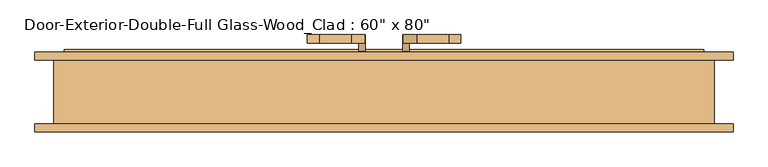
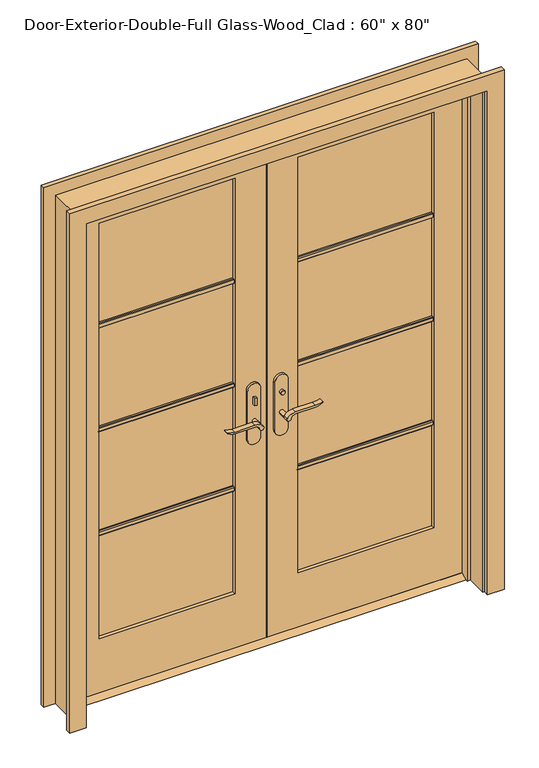
"""IFC4 building model written with IfcOpenShell, lengths in millimetres: door geometry."""

from ifc_helpers import new_model, si_unit, point, frame, frame_2d, origin, place, context, project, spatial, polyline, circle_curve, trimmed, segment, composite_curve, outline, extrude, faceted_brep, source, transform, mapped, element, save


def door_94998e6c(model_context):
    return source(origin(), model_context, "Body", "SolidModel", [
        extrude(outline(polyline([(38.1, 12.7), (73.025, 12.7), (98.425, 0.0), (12.7, 0.0), (38.1, 12.7)])), frame((-762.0, 0.0, 0.0), z_axis=(1.0, 0.0, 0.0), x_axis=(0.0, 1.0, 0.0)), (0.0, 0.0, 1.0), 1524.0),
        extrude(outline(polyline([(-47.4019111, 18.1), (-57.4019111, 18.1), (-57.4019111, 28.1), (-47.4019111, 28.1), (-47.4019111, 18.1)])), frame((0.0, 0.0, 981.9), z_axis=(0.0, 0.0, 1.0), x_axis=(1.0, 0.0, 0.0)), (0.0, 0.0, 1.0), 30.0),
        extrude(outline(composite_curve([segment(trimmed(circle_curve(frame_2d((996.9, -52.4019111)), 8.0), [point((996.9, -60.4019111))], [point((996.9, -44.4019111))], False, "CARTESIAN"), True, "CONTINUOUS"), segment(trimmed(circle_curve(frame_2d((996.9, -52.4019111)), 8.0), [point((996.9, -44.4019111))], [point((996.9, -60.4019111))], False, "CARTESIAN"), True, "CONTINUOUS")], self_intersect=False)), frame((0.0, 83.025, 0.0), z_axis=(0.0, 1.0, 0.0), x_axis=(0.0, 0.0, 1.0)), (0.0, 0.0, 1.0), 10.0),
        extrude(outline(composite_curve([segment(trimmed(circle_curve(frame_2d((897.1555521, -76.0694241)), 37.2832219), [point((919.0523287, -45.8937749))], [point((934.4, -77.7693445))], False, "CARTESIAN"), True, "CONTINUOUS"), segment(polyline([(934.4, -77.7693445), (934.4, -154.045502)]), True, "CONTINUOUS"), segment(trimmed(circle_curve(frame_2d((1017.6850638, -153.9791202)), 83.2850902), [point((934.4, -154.045502))], [point((939.4, -182.4019111))], True, "CARTESIAN"), True, "CONTINUOUS"), segment(polyline([(939.4, -182.4019111), (936.6135558, -182.4019111)]), True, "CONTINUOUS"), segment(trimmed(circle_curve(frame_2d((986.6709207, -150.4622499)), 59.3791355), [point((936.6135558, -182.4019111))], [point((927.4, -154.045502))], False, "CARTESIAN"), True, "CONTINUOUS"), segment(polyline([(927.4, -154.045502), (927.4, -77.7881013)]), True, "CONTINUOUS"), segment(trimmed(circle_curve(frame_2d((909.2738613, -77.7881013)), 18.1261387), [point((927.4, -77.7881013))], [point((914.4, -60.4019111))], True, "CARTESIAN"), True, "CONTINUOUS"), segment(trimmed(circle_curve(frame_2d((914.4, -52.4019111)), 8.0), [point((914.4, -60.4019111))], [point((919.0523287, -45.8937749))], False, "CARTESIAN"), True, "CONTINUOUS")], self_intersect=False)), frame((0.0, -21.9, 0.0), z_axis=(0.0, 1.0, 0.0), x_axis=(0.0, 0.0, 1.0)), (0.0, 0.0, 1.0), 20.0),
        extrude(outline(composite_curve([segment(trimmed(circle_curve(frame_2d((914.4, -52.4019111)), 8.0), [point((914.3999903, -60.4019111))], [point((919.0523287, -45.8937749))], False, "CARTESIAN"), True, "CONTINUOUS"), segment(trimmed(circle_curve(frame_2d((897.1555521, -76.0694241)), 37.2832219), [point((919.0523287, -45.8937749))], [point((934.4, -77.7693445))], False, "CARTESIAN"), True, "CONTINUOUS"), segment(polyline([(934.4, -77.7693445), (934.4, -154.045502)]), True, "CONTINUOUS"), segment(trimmed(circle_curve(frame_2d((1017.6850638, -153.9791202)), 83.2850902), [point((934.4, -154.045502))], [point((939.4, -182.4019111))], True, "CARTESIAN"), True, "CONTINUOUS"), segment(polyline([(939.4, -182.4019111), (936.6135558, -182.4019111)]), True, "CONTINUOUS"), segment(trimmed(circle_curve(frame_2d((986.6709207, -150.4622499)), 59.3791355), [point((936.6135558, -182.4019111))], [point((927.4, -154.045502))], False, "CARTESIAN"), True, "CONTINUOUS"), segment(polyline([(927.4, -154.045502), (927.4, -77.788099)]), True, "CONTINUOUS"), segment(trimmed(circle_curve(frame_2d((909.2738682, -77.788099)), 18.1261318), [point((927.4, -77.788099))], [point((914.3999903, -60.4019111))], True, "CARTESIAN"), True, "CONTINUOUS")], self_intersect=False)), frame((0.0, 113.025, 0.0), z_axis=(0.0, 1.0, 0.0), x_axis=(0.0, 0.0, 1.0)), (0.0, 0.0, 1.0), 20.0),
        extrude(outline(composite_curve([segment(trimmed(circle_curve(frame_2d((914.4, -52.4019111)), 8.0), [point((914.4, -60.4019111))], [point((914.4, -44.4019111))], False, "CARTESIAN"), True, "CONTINUOUS"), segment(trimmed(circle_curve(frame_2d((914.4, -52.4019111)), 8.0), [point((914.4, -44.4019111))], [point((914.4, -60.4019111))], False, "CARTESIAN"), True, "CONTINUOUS")], self_intersect=False)), frame((0.0, -1.9, 0.0), z_axis=(0.0, 1.0, 0.0), x_axis=(0.0, 0.0, 1.0)), (0.0, 0.0, 1.0), 30.0),
        extrude(outline(composite_curve([segment(trimmed(circle_curve(frame_2d((914.4, -52.4019111)), 8.0), [point((914.4, -60.4019111))], [point((914.4, -44.4019111))], False, "CARTESIAN"), True, "CONTINUOUS"), segment(trimmed(circle_curve(frame_2d((914.4, -52.4019111)), 8.0), [point((914.4, -44.4019111))], [point((914.4, -60.4019111))], False, "CARTESIAN"), True, "CONTINUOUS")], self_intersect=False)), frame((0.0, 83.025, 0.0), z_axis=(0.0, 1.0, 0.0), x_axis=(0.0, 0.0, 1.0)), (0.0, 0.0, 1.0), 30.0),
        extrude(outline(composite_curve([segment(polyline([(844.4, -27.4019111), (1039.4, -27.4019111)]), True, "CONTINUOUS"), segment(trimmed(circle_curve(frame_2d((1039.4, -52.4019111)), 25.0), [point((1039.4, -27.4019111))], [point((1039.4, -77.4019111))], False, "CARTESIAN"), True, "CONTINUOUS"), segment(polyline([(1039.4, -77.4019111), (844.4, -77.4019111)]), True, "CONTINUOUS"), segment(trimmed(circle_curve(frame_2d((844.4, -52.4019111)), 25.0), [point((844.4, -77.4019111))], [point((844.4, -27.4019111))], False, "CARTESIAN"), True, "CONTINUOUS")], self_intersect=False)), frame((0.0, 28.1, 0.0), z_axis=(0.0, 1.0, 0.0), x_axis=(0.0, 0.0, 1.0)), (0.0, 0.0, 1.0), 10.0),
        extrude(outline(composite_curve([segment(polyline([(844.4, -27.4019111), (1039.4, -27.4019111)]), True, "CONTINUOUS"), segment(trimmed(circle_curve(frame_2d((1039.4, -52.4019111)), 25.0), [point((1039.4, -27.4019111))], [point((1039.4, -77.4019111))], False, "CARTESIAN"), True, "CONTINUOUS"), segment(polyline([(1039.4, -77.4019111), (844.4, -77.4019111)]), True, "CONTINUOUS"), segment(trimmed(circle_curve(frame_2d((844.4, -52.4019111)), 25.0), [point((844.4, -77.4019111))], [point((844.4, -27.4019111))], False, "CARTESIAN"), True, "CONTINUOUS")], self_intersect=False)), frame((0.0, 73.025, 0.0), z_axis=(0.0, 1.0, 0.0), x_axis=(0.0, 0.0, 1.0)), (0.0, 0.0, 1.0), 10.0),
        extrude(outline(polyline([(47.3875, 93.025), (57.3875, 93.025), (57.3875, 83.025), (47.3875, 83.025), (47.3875, 93.025)])), frame((0.0, 0.0, 981.9), z_axis=(0.0, 0.0, 1.0), x_axis=(1.0, 0.0, 0.0)), (0.0, 0.0, 1.0), 30.0),
        extrude(outline(composite_curve([segment(trimmed(circle_curve(frame_2d((996.9, 52.3875)), 8.0), [point((996.9, 60.3875))], [point((996.9, 44.3875))], False, "CARTESIAN"), True, "CONTINUOUS"), segment(trimmed(circle_curve(frame_2d((996.9, 52.3875)), 8.0), [point((996.9, 44.3875))], [point((996.9, 60.3875))], False, "CARTESIAN"), True, "CONTINUOUS")], self_intersect=False)), frame((0.0, 18.1, 0.0), z_axis=(0.0, 1.0, 0.0), x_axis=(0.0, 0.0, 1.0)), (0.0, 0.0, 1.0), 10.0),
        extrude(outline(composite_curve([segment(trimmed(circle_curve(frame_2d((914.4, 52.3875)), 8.0), [point((919.0523287, 45.8793637))], [point((914.4, 60.3875))], False, "CARTESIAN"), True, "CONTINUOUS"), segment(trimmed(circle_curve(frame_2d((909.2738613, 77.7736901)), 18.1261387), [point((914.4, 60.3875))], [point((927.4, 77.7736901))], True, "CARTESIAN"), True, "CONTINUOUS"), segment(polyline([(927.4, 77.7736901), (927.4, 154.0310909)]), True, "CONTINUOUS"), segment(trimmed(circle_curve(frame_2d((986.6709207, 150.4478388)), 59.3791355), [point((927.4, 154.0310909))], [point((936.6135558, 182.3875))], False, "CARTESIAN"), True, "CONTINUOUS"), segment(polyline([(936.6135558, 182.3875), (939.4, 182.3875)]), True, "CONTINUOUS"), segment(trimmed(circle_curve(frame_2d((1017.6850638, 153.9647091)), 83.2850902), [point((939.4, 182.3875))], [point((934.4, 154.0310909))], True, "CARTESIAN"), True, "CONTINUOUS"), segment(polyline([(934.4, 154.0310909), (934.4, 77.7549333)]), True, "CONTINUOUS"), segment(trimmed(circle_curve(frame_2d((897.1555521, 76.0550129)), 37.2832219), [point((934.4, 77.7549333))], [point((919.0523287, 45.8793637))], False, "CARTESIAN"), True, "CONTINUOUS")], self_intersect=False)), frame((0.0, 113.025, 0.0), z_axis=(0.0, 1.0, 0.0), x_axis=(0.0, 0.0, 1.0)), (0.0, 0.0, 1.0), 20.0),
        extrude(outline(composite_curve([segment(trimmed(circle_curve(frame_2d((909.2738682, 77.7736878)), 18.1261318), [point((914.3999903, 60.3875))], [point((927.4, 77.7736878))], True, "CARTESIAN"), True, "CONTINUOUS"), segment(polyline([(927.4, 77.7736878), (927.4, 154.0310909)]), True, "CONTINUOUS"), segment(trimmed(circle_curve(frame_2d((986.6709207, 150.4478388)), 59.3791355), [point((927.4, 154.0310909))], [point((936.6135558, 182.3875))], False, "CARTESIAN"), True, "CONTINUOUS"), segment(polyline([(936.6135558, 182.3875), (939.4, 182.3875)]), True, "CONTINUOUS"), segment(trimmed(circle_curve(frame_2d((1017.6850638, 153.9647091)), 83.2850902), [point((939.4, 182.3875))], [point((934.4, 154.0310909))], True, "CARTESIAN"), True, "CONTINUOUS"), segment(polyline([(934.4, 154.0310909), (934.4, 77.7549333)]), True, "CONTINUOUS"), segment(trimmed(circle_curve(frame_2d((897.1555521, 76.0550129)), 37.2832219), [point((934.4, 77.7549333))], [point((919.0523287, 45.8793637))], False, "CARTESIAN"), True, "CONTINUOUS"), segment(trimmed(circle_curve(frame_2d((914.4, 52.3875)), 8.0), [point((919.0523287, 45.8793637))], [point((914.3999903, 60.3875))], False, "CARTESIAN"), True, "CONTINUOUS")], self_intersect=False)), frame((0.0, -21.9, 0.0), z_axis=(0.0, 1.0, 0.0), x_axis=(0.0, 0.0, 1.0)), (0.0, 0.0, 1.0), 20.0),
        extrude(outline(composite_curve([segment(trimmed(circle_curve(frame_2d((914.4, 52.3875)), 8.0), [point((914.4, 60.3875))], [point((914.4, 44.3875))], False, "CARTESIAN"), True, "CONTINUOUS"), segment(trimmed(circle_curve(frame_2d((914.4, 52.3875)), 8.0), [point((914.4, 44.3875))], [point((914.4, 60.3875))], False, "CARTESIAN"), True, "CONTINUOUS")], self_intersect=False)), frame((0.0, 83.025, 0.0), z_axis=(0.0, 1.0, 0.0), x_axis=(0.0, 0.0, 1.0)), (0.0, 0.0, 1.0), 30.0),
        extrude(outline(composite_curve([segment(trimmed(circle_curve(frame_2d((914.4, 52.3875)), 8.0), [point((914.4, 60.3875))], [point((914.4, 44.3875))], False, "CARTESIAN"), True, "CONTINUOUS"), segment(trimmed(circle_curve(frame_2d((914.4, 52.3875)), 8.0), [point((914.4, 44.3875))], [point((914.4, 60.3875))], False, "CARTESIAN"), True, "CONTINUOUS")], self_intersect=False)), frame((0.0, -1.9, 0.0), z_axis=(0.0, 1.0, 0.0), x_axis=(0.0, 0.0, 1.0)), (0.0, 0.0, 1.0), 30.0),
        extrude(outline(composite_curve([segment(trimmed(circle_curve(frame_2d((844.4, 52.3875)), 25.0), [point((844.4, 27.3875))], [point((844.4, 77.3875))], False, "CARTESIAN"), True, "CONTINUOUS"), segment(polyline([(844.4, 77.3875), (1039.4, 77.3875)]), True, "CONTINUOUS"), segment(trimmed(circle_curve(frame_2d((1039.4, 52.3875)), 25.0), [point((1039.4, 77.3875))], [point((1039.4, 27.3875))], False, "CARTESIAN"), True, "CONTINUOUS"), segment(polyline([(1039.4, 27.3875), (844.4, 27.3875)]), True, "CONTINUOUS")], self_intersect=False)), frame((0.0, 73.025, 0.0), z_axis=(0.0, 1.0, 0.0), x_axis=(0.0, 0.0, 1.0)), (0.0, 0.0, 1.0), 10.0),
        extrude(outline(composite_curve([segment(trimmed(circle_curve(frame_2d((844.4, 52.3875)), 25.0), [point((844.4, 27.3875))], [point((844.4, 77.3875))], False, "CARTESIAN"), True, "CONTINUOUS"), segment(polyline([(844.4, 77.3875), (1039.4, 77.3875)]), True, "CONTINUOUS"), segment(trimmed(circle_curve(frame_2d((1039.4, 52.3875)), 25.0), [point((1039.4, 77.3875))], [point((1039.4, 27.3875))], False, "CARTESIAN"), True, "CONTINUOUS"), segment(polyline([(1039.4, 27.3875), (844.4, 27.3875)]), True, "CONTINUOUS")], self_intersect=False)), frame((0.0, 28.1, 0.0), z_axis=(0.0, 1.0, 0.0), x_axis=(0.0, 0.0, 1.0)), (0.0, 0.0, 1.0), 10.0),
        extrude(outline(polyline([(52.07, 1502.171875), (52.07, 1483.121875), (45.72, 1483.121875), (42.545, 1486.296875), (42.545, 1498.996875), (45.72, 1502.171875), (52.07, 1502.171875)])), frame((120.65, 0.0, 0.0), z_axis=(1.0, 0.0, 0.0), x_axis=(0.0, 1.0, 0.0)), (0.0, 0.0, 1.0), 520.7),
        extrude(outline(polyline([(52.07, 1081.88125), (52.07, 1062.83125), (45.72, 1062.83125), (42.545, 1066.00625), (42.545, 1078.70625), (45.72, 1081.88125), (52.07, 1081.88125)])), frame((120.65, 0.0, 0.0), z_axis=(1.0, 0.0, 0.0), x_axis=(0.0, 1.0, 0.0)), (0.0, 0.0, 1.0), 520.7),
        extrude(outline(polyline([(52.07, 661.590625), (52.07, 642.540625), (45.72, 642.540625), (42.545, 645.715625), (42.545, 658.415625), (45.72, 661.590625), (52.07, 661.590625)])), frame((120.65, 0.0, 0.0), z_axis=(1.0, 0.0, 0.0), x_axis=(0.0, 1.0, 0.0)), (0.0, 0.0, 1.0), 520.7),
        extrude(outline(polyline([(59.055, 1502.171875), (65.405, 1502.171875), (68.58, 1498.996875), (68.58, 1486.296875), (65.405, 1483.121875), (59.055, 1483.121875), (59.055, 1502.171875)])), frame((-641.35, 0.0, 0.0), z_axis=(1.0, 0.0, 0.0), x_axis=(0.0, 1.0, 0.0)), (0.0, 0.0, 1.0), 520.7),
        extrude(outline(polyline([(59.055, 1081.88125), (65.405, 1081.88125), (68.58, 1078.70625), (68.58, 1066.00625), (65.405, 1062.83125), (59.055, 1062.83125), (59.055, 1081.88125)])), frame((-641.35, 0.0, 0.0), z_axis=(1.0, 0.0, 0.0), x_axis=(0.0, 1.0, 0.0)), (0.0, 0.0, 1.0), 520.7),
        extrude(outline(polyline([(59.055, 661.590625), (65.405, 661.590625), (68.58, 658.415625), (68.58, 645.715625), (65.405, 642.540625), (59.055, 642.540625), (59.055, 661.590625)])), frame((-641.35, 0.0, 0.0), z_axis=(1.0, 0.0, 0.0), x_axis=(0.0, 1.0, 0.0)), (0.0, 0.0, 1.0), 520.7),
        extrude(outline(polyline([(59.055, 1502.171875), (65.405, 1502.171875), (68.58, 1498.996875), (68.58, 1486.296875), (65.405, 1483.121875), (59.055, 1483.121875), (59.055, 1502.171875)])), frame((120.65, 0.0, 0.0), z_axis=(1.0, 0.0, 0.0), x_axis=(0.0, 1.0, 0.0)), (0.0, 0.0, 1.0), 520.7),
        extrude(outline(polyline([(59.055, 1081.88125), (65.405, 1081.88125), (68.58, 1078.70625), (68.58, 1066.00625), (65.405, 1062.83125), (59.055, 1062.83125), (59.055, 1081.88125)])), frame((120.65, 0.0, 0.0), z_axis=(1.0, 0.0, 0.0), x_axis=(0.0, 1.0, 0.0)), (0.0, 0.0, 1.0), 520.7),
        extrude(outline(polyline([(59.055, 661.590625), (65.405, 661.590625), (68.58, 658.415625), (68.58, 645.715625), (65.405, 642.540625), (59.055, 642.540625), (59.055, 661.590625)])), frame((120.65, 0.0, 0.0), z_axis=(1.0, 0.0, 0.0), x_axis=(0.0, 1.0, 0.0)), (0.0, 0.0, 1.0), 520.7),
        extrude(outline(polyline([(52.07, 1502.171875), (52.07, 1483.121875), (45.72, 1483.121875), (42.545, 1486.296875), (42.545, 1498.996875), (45.72, 1502.171875), (52.07, 1502.171875)])), frame((-641.35, 0.0, 0.0), z_axis=(1.0, 0.0, 0.0), x_axis=(0.0, 1.0, 0.0)), (0.0, 0.0, 1.0), 520.7),
        extrude(outline(polyline([(52.07, 1081.88125), (52.07, 1062.83125), (45.72, 1062.83125), (42.545, 1066.00625), (42.545, 1078.70625), (45.72, 1081.88125), (52.07, 1081.88125)])), frame((-641.35, 0.0, 0.0), z_axis=(1.0, 0.0, 0.0), x_axis=(0.0, 1.0, 0.0)), (0.0, 0.0, 1.0), 520.7),
        extrude(outline(polyline([(52.07, 661.590625), (52.07, 642.540625), (45.72, 642.540625), (42.545, 645.715625), (42.545, 658.415625), (45.72, 661.590625), (52.07, 661.590625)])), frame((-641.35, 0.0, 0.0), z_axis=(1.0, 0.0, 0.0), x_axis=(0.0, 1.0, 0.0)), (0.0, 0.0, 1.0), 520.7),
        extrude(outline(polyline([(0.0, 768.35), (0.0, 831.85), (2101.85, 831.85), (2101.85, -831.85), (0.0, -831.85), (0.0, -768.35), (2038.35, -768.35), (2038.35, 768.35), (0.0, 768.35)])), frame((0.0, 73.025, 0.0), z_axis=(0.0, 1.0, 0.0), x_axis=(0.0, 0.0, 1.0)), (0.0, 0.0, 1.0), 19.05),
        extrude(outline(polyline([(0.0, 768.35), (0.0, 831.85), (2101.85, 831.85), (2101.85, -831.85), (0.0, -831.85), (0.0, -768.35), (2038.35, -768.35), (2038.35, 768.35), (0.0, 768.35)])), frame((0.0, -98.425, 0.0), z_axis=(0.0, 1.0, 0.0), x_axis=(0.0, 0.0, 1.0)), (0.0, 0.0, 1.0), 19.05),
        extrude(outline(polyline([(12.7, 762.0), (2032.0, 762.0), (2032.0, 1.5875), (12.7, 1.5875), (12.7, 762.0)]), holes=[polyline([(1912.9375, 120.65), (1912.9375, 641.35), (231.775, 641.35), (231.775, 120.65), (1912.9375, 120.65)])]), frame((0.0, 38.1, 0.0), z_axis=(0.0, 1.0, 0.0), x_axis=(0.0, 0.0, 1.0)), (0.0, 0.0, 1.0), 34.925),
        extrude(outline(polyline([(2032.0, -762.0), (12.7, -762.0), (12.7, -1.6019111), (2032.0, -1.6019111), (2032.0, -762.0)]), holes=[polyline([(231.775, -641.35), (1912.9375, -641.35), (1912.9375, -120.65), (231.775, -120.65), (231.775, -641.35)])]), frame((0.0, 38.1, 0.0), z_axis=(0.0, 1.0, 0.0), x_axis=(0.0, 0.0, 1.0)), (0.0, 0.0, 1.0), 34.925),
        faceted_brep([(787.4, 73.025, 0.0), (787.4, -79.375, 0.0), (762.0, -79.375, 0.0), (762.0, 3.175, 0.0), (749.3, 3.175, 0.0), (749.3, 38.1, 0.0), (762.0, 38.1, 0.0), (762.0, 73.025, 0.0), (787.4, 73.025, 2057.4), (787.4, -79.375, 2057.4), (-787.4, -79.375, 2057.4), (-787.4, -79.375, 0.0), (-762.0, -79.375, 0.0), (-762.0, -79.375, 2032.0), (762.0, -79.375, 2032.0), (762.0, 3.175, 2032.0), (-762.0, 3.175, 2032.0), (-762.0, 3.175, 0.0), (-749.3, 3.175, 0.0), (-749.3, 3.175, 2019.3), (749.3, 3.175, 2019.3), (749.3, 38.1, 2019.3), (1.5875, 38.1, 2019.3), (-1.6019111, 38.1, 2019.3), (-749.3, 38.1, 2019.3), (-749.3, 38.1, 0.0), (-762.0, 38.1, 0.0), (-762.0, 38.1, 2032.0), (-1.6019111, 38.1, 2032.0), (1.5875, 38.1, 2032.0), (762.0, 38.1, 2032.0), (762.0, 73.025, 2032.0), (1.5875, 73.025, 2032.0), (-1.6019111, 73.025, 2032.0), (-762.0, 73.025, 2032.0), (-762.0, 73.025, 0.0), (-787.4, 73.025, 0.0), (-787.4, 73.025, 2057.4)], [[[0, 1, 2, 3, 4, 5, 6, 7]], [[1, 0, 8, 9]], [[2, 1, 9, 10, 11, 12, 13, 14]], [[3, 2, 14, 15]], [[4, 3, 15, 16, 17, 18, 19, 20]], [[5, 4, 20, 21]], [[6, 5, 21, 22, 23, 24, 25, 26, 27, 28, 29, 30]], [[7, 6, 30, 31]], [[0, 7, 31, 32, 33, 34, 35, 36, 37, 8]], [[9, 8, 37, 10]], [[14, 13, 16, 15]], [[20, 19, 24, 23, 22, 21]], [[31, 30, 29, 28, 27, 34, 33, 32]], [[12, 11, 36, 35, 26, 25, 18, 17]], [[11, 10, 37, 36]], [[13, 12, 17, 16]], [[19, 18, 25, 24]], [[27, 26, 35, 34]]]),
        extrude(outline(polyline([(641.35, 52.07), (120.65, 52.07), (120.65, 59.055), (641.35, 59.055), (641.35, 52.07)])), frame((0.0, 0.0, 231.775), z_axis=(0.0, 0.0, 1.0), x_axis=(1.0, 0.0, 0.0)), (0.0, 0.0, 1.0), 1681.1625),
        extrude(outline(polyline([(-120.65, 52.07), (-641.35, 52.07), (-641.35, 59.055), (-120.65, 59.055), (-120.65, 52.07)])), frame((0.0, 0.0, 231.775), z_axis=(0.0, 0.0, 1.0), x_axis=(1.0, 0.0, 0.0)), (0.0, 0.0, 1.0), 1681.1625),
    ])


if __name__ == "__main__":
    model = new_model("IFC4")
    model_context = context("Model", 3, world=origin())
    ifc_project = project(units=[si_unit("LENGTHUNIT", "METRE", prefix="MILLI")], contexts=[model_context])
    site = spatial("IfcSite", under=ifc_project)
    building = spatial("IfcBuilding", under=site)
    placement = place(None, origin())
    door_shape = door_94998e6c(model_context)
    element("IfcDoor", 1, ObjectType="Door-Exterior-Double-Full Glass-Wood_Clad : 60\" x 80\"", at=placement, inside=building, context=model_context, shape_type="MappedRepresentation", body=[
        mapped(door_shape, transform((0.0, 0.0, 0.0), x_axis=(1.0, 0.0, 0.0), y_axis=(0.0, 1.0, 0.0), z_axis=(0.0, 0.0, 1.0))),
    ])
    save(model, "model.ifc")

# Revit data of these elements
# Type "Door-Exterior-Double-Full Glass-Wood_Clad : 60\" x 80\""
#   Type Mark = "12"
#   Assembly Code = "B2030100"
#   Analytic Construction = "French door, wood frame with double glass"
#   Top Rail = 0' - 4 11/16"
#   Threshold Offset [instance default] = 0' - 0 1/2"
#   Thickness = 0' - 1 3/8"
#   Thermal Resistance (R) = 1.9158 (h·ft²·°F)/BTU
#   Swing Angle [instance default] = 90.00°
#   Stiles = 0' - 4 3/4"
#   Rough Width = 5' - 2"
#   Rough Height = 6' - 9"
#   Panel Width = 2' - 6"
#   Door Offset [instance default] = 0' - 0"
#   Height = 6' - 8"
#   Width = 5' - 0"
#   Heat Transfer Coefficient (U) = 0.5220 BTU/(h·ft²·°F)
#   Bottom Rail = 0' - 9 1/8"
#   Exterior Trim [instance default] = yes
#   Threshold [instance default] = yes
#   Show Grill [instance default] = yes
#   Function = 1
#   Trim Material = Cherry
#   Threshold Material = Cherry
#   Panel Material = Cherry
#   Glazing = Glass
#   Frame Material = Cherry
#   Door Handle Material = Aluminum
#   Visual Light Transmittance = 0
#   Solar Heat Gain Coefficient = 0
#   Wall Closure = (empty or 0)
#   Construction Type = (empty or 0)
# Element 1 (IfcDoor, "Door-Exterior-Double-Full Glass-Wood_Clad : 60\" x 80\"")
#   Materials on its faces: "Cherry", "Aluminum", "Glass"
# Materials
#   "Cherry": class "Wood", colour RGB 226 177 128, transparency 0, Description = "Prunus Serotina", Cost = 0
#   "Glass": class "Glass", colour RGB 0 128 192, transparency 0.75, Description = "Soda Lime Glass", Cost = 0
#   "Aluminum": class "Metal", colour RGB 247 247 247, transparency 0, Description = "Aluminum 6061", Cost = 0
